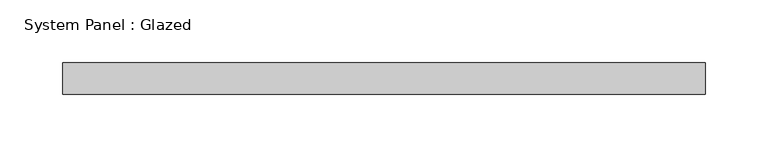
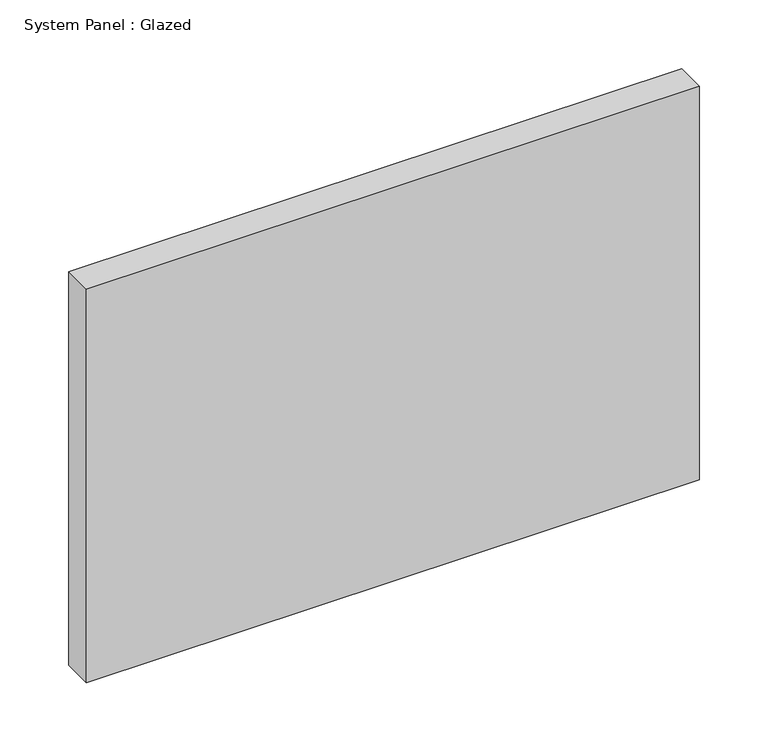
"""IFC4 building model written with IfcOpenShell, lengths in millimetres: plate geometry, System Panel : Glazed."""

from ifc_helpers import new_model, si_unit, origin, origin_with_axes, place, context, project, spatial, polyline, outline, extrude, source, transform, mapped, element, save


def system_panel_glazed_055f9577(model_context):
    return source(origin(), model_context, "Body", "SweptSolid", [
        extrude(outline(polyline([(257.175, 19.05), (-257.175, 19.05), (-257.175, 44.45), (257.175, 44.45), (257.175, 19.05)])), origin_with_axes(), (0.0, 0.0, 1.0), 349.25),
    ])


if __name__ == "__main__":
    model = new_model("IFC4")
    model_context = context("Model", 3, world=origin())
    ifc_project = project(units=[si_unit("LENGTHUNIT", "METRE", prefix="MILLI")], contexts=[model_context])
    site = spatial("IfcSite", under=ifc_project)
    building = spatial("IfcBuilding", under=site)
    placement = place(None, origin())
    system_panel_glazed_shape = system_panel_glazed_055f9577(model_context)
    element("IfcPlate", 1, ObjectType="System Panel : Glazed", at=placement, inside=building, context=model_context, shape_type="MappedRepresentation", body=[
        mapped(system_panel_glazed_shape, transform((0.0, 0.0, 0.0), x_axis=(1.0, 0.0, 0.0), y_axis=(0.0, 1.0, 0.0), z_axis=(0.0, 0.0, 1.0))),
    ])
    save(model, "model.ifc")

# Revit data of these elements
# Type "System Panel : Glazed"
#   Construction Type Id = "GSP4R"
#   Analytic Construction = "1/8 in Pilkington single glazing"
#   Visual Light Transmittance = 0.9
#   Solar Heat Gain Coefficient = 0.86
#   Heat Transfer Coefficient (U) = 1.18115 BTU/(h·ft²·°F)
#   Define Thermal Properties by = 1
# Element 1 (IfcPlate, "System Panel : Glazed")
#   Materials on its faces: "Glass"
# Materials
#   "Glass": class "Glass", colour RGB 0 128 192, transparency 0.75, Description = "Soda Lime Glass", Cost = 0
